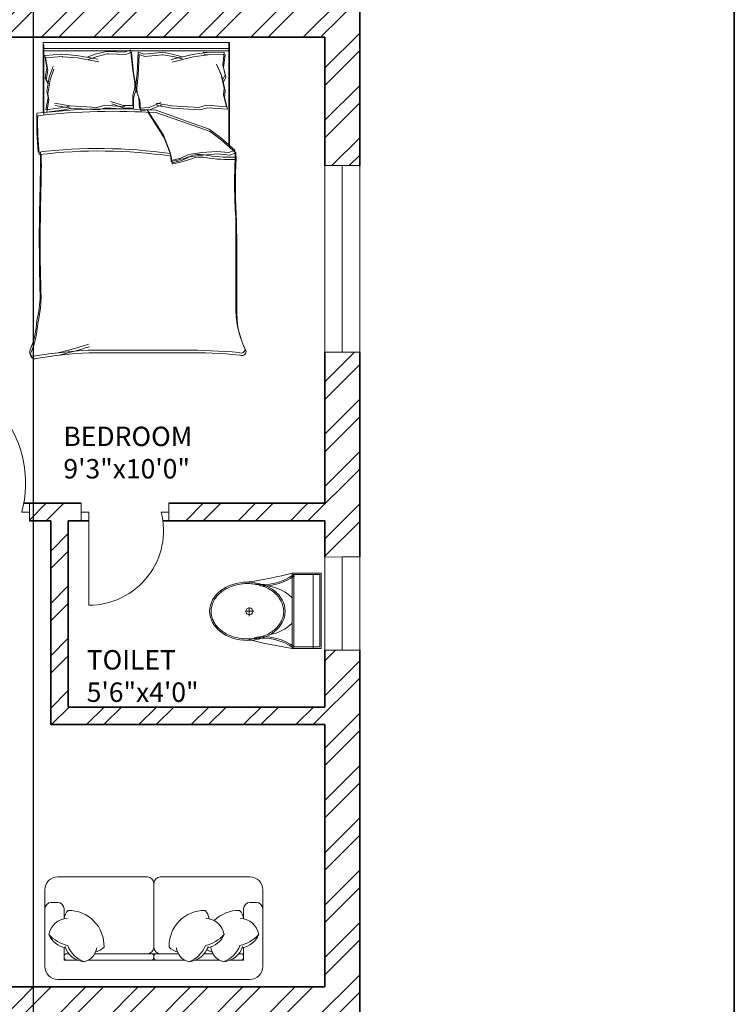
# Model space of a CAD drawing. Units: inches. Extents: x 2552 to 3217, y 1417 to 2737.
# Tile 6 of 25: x 3033 to 3217, y 1631 to 1885. Entities that reach past the tile are written whole.
import ezdxf

# ---------------------------------------------------------------- set-up
doc = ezdxf.new("R2010")
doc.units = ezdxf.units.IN
for name, color, linetype, lineweight in [('A-ANNO-DIMS', 2, 'Continuous', 18), ('A-ANNO-TTLB', 7, 'Continuous', 35), ('A-AREA-IDEN', 7, 'Continuous', 18), ('A-DOOR', 21, 'Continuous', 18), ('A-FLOR-FIXT', 8, 'Continuous', 18), ('A-FURN', 8, 'Continuous', 13), ('A-GLAZ', 161, 'Continuous', 18), ('A-WALL', 7, 'Continuous', 35), ('A-WALL-PATT', 217, 'Continuous', 13)]:
    doc.layers.add(name, color=color, linetype=linetype, lineweight=lineweight)
doc.styles.get("Standard").update_dxf_attribs({"font": 'arial.ttf'})
doc.dimstyles.get("Standard").update_dxf_attribs({"dimtxt": 0.18, "dimasz": 0.18, "dimexe": 0.18, "dimexo": 0.0625, "dimgap": 0.09, "dimtad": 0, "dimtih": 1, "dimtoh": 1, "dimdec": 4, "dimzin": 0, "dimdsep": 46, "dimtxsty": 'Standard', "dimcen": 0.09, "dimadec": 0, "dimazin": 0, "dimtfac": 1, "dimtdec": 4, "dimtofl": 0, "dimtmove": 0, "dimatfit": 3, "dimfxl": 1, "dimtolj": 1, "dimtzin": 0, "dimarcsym": 0})

# ---------------------------------------------------------------- blocks, each defined once
blk = doc.blocks.new('A$C31115884')
for p, q in [((283.1, 497.7), (223.4, 497.7)), ((257.5, 466.4), (257.5, 523.2)), ((0, 200), (0, 0)), ((520, 200), (0, 200)), ((10, 190), (10, 10)), ((510, 190), (10, 190)), ((510, 10), (510, 190)), ((520, 0), (520, 200)), ((510, 54.5), (0, 54.5)), ((10, 10), (510, 10)), ((0, 0), (520, 0))]:
    blk.add_line(p, q)
blk.add_circle((255.6, 496.4), 23.6)
for centre, radius, start, end in [((2777.7, -204.6), 2807, 165.4549, 171.71327), ((3237, 905), 2807, 188.28673, 194.5451), ((-294.5, 403.3), 364.7, 324.20913, 9.34987), ((-294.5, 403.3), 374.7, 324.20913, 9.34987), ((139.5, 406.2), 293.5, 315.84364, 2.65635), ((805.8, 403.3), 374.7, 179.20365, 215.79087), ((805.8, 403.3), 364.7, 170.65013, 215.79087), ((383.6, 406.2), 293.5, 190.27735, 224.15636)]:
    blk.add_arc(centre, radius, start, end)
blk.add_ellipse((256.2, 509.9), major_axis=(0, -260.7), ratio=0.772727)
blk.add_open_spline([(256.2, 259.2), (263.1, 259.2), (270, 259.7), (287.8, 262.3), (298.7, 265.1), (319.9, 273.1), (330.2, 278.4), (350.1, 291.1), (359.7, 298.7), (377.7, 315.9), (386.2, 325.5), (401.7, 346.6), (408.8, 358.1), (421.3, 382.5), (426.8, 395.5), (435.9, 422.4), (439.5, 436.4), (444.8, 465.1), (446.5, 479.7), (447.9, 509.2), (447.6, 524), (445, 553.3), (442.7, 567.8), (436.3, 596), (432.1, 609.7), (421.9, 636), (416, 648.6), (402.5, 672.1), (395, 683), (378.6, 703), (369.8, 712.1), (351.1, 728), (341.3, 734.8), (320.9, 746.2), (310.4, 750.7), (288.9, 757.3), (278, 759.4), (256, 761), (245, 760.6), (223.1, 757.2), (212.3, 754.3), (191.1, 746.1), (180.8, 740.7), (160.9, 727.8), (151.4, 720.1), (133.5, 702.7), (125.1, 693), (109.6, 671.7), (102.6, 660.2), (90.2, 635.7), (84.9, 622.7), (76, 595.6), (72.4, 581.6), (67.2, 552.9), (65.6, 538.2), (64.4, 508.8), (64.8, 494), (67.5, 464.7), (69.9, 450.2), (76.6, 422), (80.8, 408.3), (91.1, 382.2), (97.2, 369.7), (110.8, 346.3), (118.4, 335.4), (134.8, 315.6), (143.7, 306.7), (162.4, 290.9), (172.3, 284.2), (192.8, 273), (203.3, 268.6), (224.8, 262.2), (235.8, 260.2), (249.9, 259.3), (253, 259.2), (256.2, 259.2)], degree=3, knots=[0, 0, 0, 0, 0.110105, 0.110105, 0.285049, 0.285049, 0.459994, 0.459994, 0.634938, 0.634938, 0.809882, 0.809882, 0.984827, 0.984827, 1.159771, 1.159771, 1.334715, 1.334715, 1.50966, 1.50966, 1.684604, 1.684604, 1.859549, 1.859549, 2.034493, 2.034493, 2.209437, 2.209437, 2.384382, 2.384382, 2.559326, 2.559326, 2.73427, 2.73427, 2.909215, 2.909215, 3.084159, 3.084159, 3.259103, 3.259103, 3.434048, 3.434048, 3.608992, 3.608992, 3.783936, 3.783936, 3.958881, 3.958881, 4.133825, 4.133825, 4.30877, 4.30877, 4.483714, 4.483714, 4.658658, 4.658658, 4.833603, 4.833603, 5.008547, 5.008547, 5.183491, 5.183491, 5.358436, 5.358436, 5.53338, 5.53338, 5.708324, 5.708324, 5.883269, 5.883269, 6.058213, 6.058213, 6.233158, 6.233158, 6.283185, 6.283185, 6.283185, 6.283185])
blk = doc.blocks.new('BED-DOUBLE')
for p, q in [((3.47, 63.33), (3.47, 81.44)), ((3.47, 81.44), (51.49, 81.44)), ((3.48, 63.33), (3.48, 81.44)), ((51.27, 81.44), (51.27, 54.83)), ((51.27, 81.44), (51.27, 54.83)), ((51.49, 81.44), (51.49, 80.8)), ((3.47, 79.91), (51.27, 79.91)), ((3.48, 79.91), (51.27, 79.91)), ((3.7, 62.69), (3.7, 80.8)), ((3.7, 62.69), (3.7, 80.8)), ((3.7, 79.27), (51.49, 79.27)), ((3.7, 79.27), (51.49, 79.27)), ((16.88, 78.42), (19.77, 79.14)), ((16.88, 78.42), (19.77, 79.14)), ((19.77, 79.14), (20.09, 79.14)), ((19.77, 79.14), (20.09, 79.14)), ((20.09, 79.14), (24.54, 78.99)), ((20.09, 79.14), (24.54, 78.99)), ((24.54, 78.99), (25.98, 79.57)), ((24.54, 78.99), (25.98, 79.57)), ((24.77, 78.36), (26.21, 78.93)), ((24.77, 78.36), (26.21, 78.93)), ((25.98, 79.57), (26.56, 74.22)), ((25.98, 79.57), (26.56, 74.22)), ((26.21, 78.93), (26.79, 73.58)), ((26.21, 78.93), (26.79, 73.58)), ((27.98, 78.95), (27.73, 73.58)), ((27.98, 78.95), (27.73, 73.58)), ((29.46, 78.46), (27.98, 78.95)), ((29.46, 78.46), (27.98, 78.95)), ((33.88, 78.89), (29.46, 78.46)), ((33.88, 78.89), (29.46, 78.46)), ((34.2, 78.91), (33.88, 78.89)), ((34.2, 78.91), (33.88, 78.89)), ((37.14, 78.36), (34.2, 78.91)), ((37.14, 78.36), (34.2, 78.91)), ((45.71, 78.9), (41.91, 78.37)), ((45.71, 78.9), (41.91, 78.37)), ((50.11, 78.89), (44.71, 78.98)), ((44.71, 78.98), (45.71, 78.9)), ((50.11, 78.89), (44.71, 78.98)), ((44.71, 78.98), (45.71, 78.9)), ((50.11, 78.89), (49.73, 75.68)), ((50.11, 78.89), (49.73, 75.68)), ((51.49, 80.8), (51.49, 54.19)), ((51.49, 80.8), (51.49, 54.19)), ((3.89, 78.13), (4.47, 74.95)), ((3.89, 78.13), (4.47, 74.95)), ((3.9, 78.11), (8.18, 78.43)), ((3.9, 78.11), (8.18, 78.43)), ((4.12, 77.49), (4.7, 74.31)), ((4.12, 77.49), (4.7, 74.31)), ((4.13, 77.47), (8.41, 77.8)), ((4.13, 77.47), (8.41, 77.8)), ((8.18, 78.43), (8.28, 78.42)), ((8.18, 78.43), (8.28, 78.42)), ((8.28, 78.42), (12.11, 78.13)), ((8.28, 78.42), (12.11, 78.13)), ((8.41, 77.8), (8.51, 77.78)), ((8.41, 77.8), (8.51, 77.78)), ((8.51, 77.78), (12.34, 77.49)), ((8.51, 77.78), (12.34, 77.49)), ((12.11, 78.13), (17.6, 77.12)), ((12.11, 78.13), (17.6, 77.12)), ((12.34, 77.49), (17.83, 76.48)), ((12.34, 77.49), (17.83, 76.48)), ((14.85, 77.69), (16.88, 78.42)), ((14.85, 77.69), (16.88, 78.42)), ((15.08, 77.05), (17.11, 77.78)), ((15.08, 77.05), (17.11, 77.78)), ((17.11, 77.78), (20, 78.5)), ((17.11, 77.78), (20, 78.5)), ((20, 78.5), (20.32, 78.5)), ((20, 78.5), (20.32, 78.5)), ((20.32, 78.5), (24.77, 78.36)), ((20.32, 78.5), (24.77, 78.36)), ((28.21, 78.31), (27.96, 72.94)), ((28.21, 78.31), (27.96, 72.94)), ((29.68, 77.83), (28.21, 78.31)), ((29.68, 77.83), (28.21, 78.31)), ((34.11, 78.25), (29.68, 77.83)), ((34.11, 78.25), (29.68, 77.83)), ((34.43, 78.27), (34.11, 78.25)), ((34.43, 78.27), (34.11, 78.25)), ((37.36, 77.73), (34.43, 78.27)), ((37.36, 77.73), (34.43, 78.27)), ((41.91, 78.37), (36.49, 77.02)), ((41.91, 78.37), (36.5, 77.02)), ((42.14, 77.73), (36.72, 76.38)), ((42.14, 77.73), (36.72, 76.38)), ((39.2, 77.77), (37.14, 78.36)), ((39.2, 77.77), (37.14, 78.36)), ((39.43, 77.13), (37.36, 77.73)), ((39.43, 77.13), (37.36, 77.73)), ((45.94, 78.26), (42.14, 77.73)), ((45.94, 78.26), (42.14, 77.73)), ((50.34, 78.25), (44.94, 78.34)), ((44.94, 78.34), (45.94, 78.26)), ((50.34, 78.25), (44.94, 78.34)), ((44.94, 78.34), (45.94, 78.26)), ((50.34, 78.25), (49.96, 75.04)), ((50.34, 78.25), (49.96, 75.04)), ((4.47, 74.95), (4.04, 72.34)), ((4.47, 74.95), (4.04, 72.34)), ((4.7, 74.31), (4.27, 71.7)), ((4.7, 74.31), (4.27, 71.7)), ((5.05, 72.49), (6.06, 75.24)), ((5.05, 72.49), (6.06, 75.24)), ((5.28, 71.85), (6.29, 74.6)), ((5.28, 71.85), (6.29, 74.6)), ((26.56, 74.22), (27.14, 71.04)), ((26.56, 74.22), (27.14, 71.04)), ((26.79, 73.58), (27.37, 70.4)), ((26.79, 73.58), (27.37, 70.4)), ((27.73, 73.58), (27.35, 70.37)), ((27.73, 73.58), (27.35, 70.37)), ((49.31, 73.19), (48.13, 75.86)), ((49.31, 73.19), (48.13, 75.86)), ((49.54, 72.55), (48.36, 75.23)), ((49.54, 72.55), (48.36, 75.23)), ((49.73, 75.68), (50.33, 73.1)), ((49.73, 75.68), (50.33, 73.1)), ((49.96, 75.04), (50.56, 72.47)), ((49.96, 75.04), (50.56, 72.47)), ((4.04, 72.34), (4.62, 71.33)), ((4.04, 72.34), (4.62, 71.33)), ((4.27, 71.7), (4.85, 70.69)), ((4.27, 71.7), (4.85, 70.69)), ((4.47, 68.87), (5.05, 72.49)), ((4.47, 68.87), (5.05, 72.49)), ((4.7, 68.23), (5.28, 71.85)), ((4.7, 68.23), (5.28, 71.85)), ((27.14, 71.04), (27.14, 69.74)), ((27.14, 71.04), (27.14, 69.74)), ((27.96, 72.94), (27.58, 69.73)), ((27.96, 72.94), (27.58, 69.73)), ((50.11, 69.61), (49.31, 73.19)), ((50.11, 69.61), (49.31, 73.19)), ((50.34, 68.98), (49.54, 72.55)), ((50.34, 68.98), (49.54, 72.55)), ((50.33, 73.1), (49.81, 72.06)), ((50.33, 73.1), (49.81, 72.06)), ((50.56, 72.47), (50.04, 71.42)), ((50.56, 72.47), (50.04, 71.42)), ((4.76, 67.28), (4.47, 68.87)), ((4.76, 67.28), (4.47, 68.87)), ((27.14, 69.74), (26.56, 67.86)), ((27.14, 69.74), (26.56, 67.86)), ((27.37, 69.1), (26.79, 67.22)), ((27.37, 69.1), (26.79, 67.22)), ((27.35, 70.37), (27.44, 69.07)), ((27.35, 70.37), (27.44, 69.07)), ((27.37, 70.4), (27.37, 69.1)), ((27.37, 70.4), (27.37, 69.1)), ((27.44, 69.07), (28.13, 67.23)), ((27.44, 69.07), (28.13, 67.23)), ((27.58, 69.73), (27.66, 68.43)), ((27.58, 69.73), (27.66, 68.43)), ((49.92, 68.01), (50.11, 69.61)), ((49.92, 68.01), (50.11, 69.61)), ((50.15, 67.37), (50.34, 68.98)), ((50.15, 67.37), (50.34, 68.98)), ((4.18, 64.1), (4.76, 67.28)), ((4.18, 64.1), (4.76, 67.28)), ((4.41, 63.46), (4.99, 66.64)), ((4.41, 63.46), (4.99, 66.64)), ((4.99, 66.64), (4.7, 68.23)), ((4.99, 66.64), (4.7, 68.23)), ((24.1, 65.18), (20.96, 66.27)), ((24.1, 65.18), (20.96, 66.27)), ((26.56, 67.86), (26.56, 65.18)), ((26.56, 67.86), (26.56, 65.18)), ((26.79, 67.22), (26.79, 64.54)), ((26.79, 67.22), (26.79, 64.54)), ((27.66, 68.43), (28.36, 66.59)), ((27.66, 68.43), (28.36, 66.59)), ((28.13, 67.23), (28.3, 64.55)), ((28.13, 67.23), (28.3, 64.55)), ((28.36, 66.59), (28.53, 63.91)), ((28.36, 66.59), (28.53, 63.91)), ((30.75, 64.7), (33.82, 65.99)), ((30.75, 64.7), (33.82, 65.99)), ((50.7, 64.87), (49.92, 68.01)), ((50.7, 64.87), (49.92, 68.01)), ((50.93, 64.23), (50.15, 67.37)), ((50.93, 64.23), (50.15, 67.37)), ((9.28, 64.83), (4.18, 64.1)), ((9.28, 64.83), (4.18, 64.1)), ((9.51, 64.19), (4.41, 63.46)), ((9.51, 64.19), (4.41, 63.46)), ((6.38, 65.81), (10.41, 65.15)), ((6.38, 65.81), (10.41, 65.15)), ((6.61, 65.18), (10.64, 64.51)), ((6.61, 65.18), (10.64, 64.51)), ((10.41, 65.15), (9.28, 64.83)), ((10.41, 65.15), (9.28, 64.83)), ((10.64, 64.51), (9.51, 64.19)), ((10.64, 64.51), (9.51, 64.19)), ((10.41, 65.15), (17.42, 64.72)), ((10.41, 65.15), (17.42, 64.72)), ((10.64, 64.51), (17.65, 64.08)), ((10.64, 64.51), (17.65, 64.08)), ((17.42, 64.72), (19.38, 65.27)), ((17.42, 64.72), (19.38, 65.27)), ((17.65, 64.08), (19.61, 64.63)), ((17.65, 64.08), (19.61, 64.63)), ((19.38, 65.27), (24.52, 64.87)), ((19.38, 65.27), (24.52, 64.87)), ((19.61, 64.63), (24.74, 64.23)), ((19.61, 64.63), (24.74, 64.23)), ((24.33, 64.54), (21.19, 65.63)), ((24.33, 64.54), (21.19, 65.63)), ((26.56, 65.18), (24.1, 65.18)), ((26.56, 65.18), (24.1, 65.18)), ((26.79, 64.54), (24.33, 64.54)), ((26.79, 64.54), (24.33, 64.54)), ((28.3, 64.55), (30.75, 64.7)), ((28.3, 64.55), (30.75, 64.7)), ((28.53, 63.91), (30.98, 64.06)), ((28.53, 63.91), (30.98, 64.06)), ((30.26, 64.06), (34.45, 57.57)), ((30.26, 64.06), (34.45, 57.57)), ((30.49, 63.42), (34.68, 56.93)), ((30.49, 63.42), (34.68, 56.93)), ((30.98, 64.06), (34.05, 65.35)), ((30.98, 64.06), (34.05, 65.35)), ((40.64, 61.13), (32.31, 64.06)), ((40.64, 61.13), (32.31, 64.06)), ((40.87, 60.49), (32.53, 63.42)), ((40.87, 60.49), (32.53, 63.42)), ((32.56, 65.81), (36.6, 65.15)), ((32.56, 65.81), (36.6, 65.15)), ((32.79, 65.18), (36.82, 64.51)), ((32.79, 65.18), (36.82, 64.51)), ((36.6, 65.15), (43.61, 64.72)), ((36.6, 65.15), (43.61, 64.72)), ((36.82, 64.51), (43.83, 64.08)), ((36.82, 64.51), (43.83, 64.08)), ((43.61, 64.72), (45.57, 65.27)), ((43.61, 64.72), (45.57, 65.27)), ((43.83, 64.08), (45.79, 64.63)), ((43.83, 64.08), (45.79, 64.63)), ((45.57, 65.27), (50.7, 64.87)), ((45.57, 65.27), (50.7, 64.87)), ((45.79, 64.63), (50.93, 64.23)), ((45.79, 64.63), (50.93, 64.23)), ((46.22, 59.11), (40.64, 61.13)), ((46.22, 59.11), (40.64, 61.13)), ((46.45, 58.48), (40.87, 60.49)), ((46.45, 58.48), (40.87, 60.49)), ((49.16, 56.95), (46.22, 59.11)), ((49.16, 56.95), (46.22, 59.11)), ((49.39, 56.31), (46.45, 58.48)), ((49.39, 56.31), (46.45, 58.48)), ((34.45, 57.57), (36.15, 53.08)), ((34.45, 57.57), (36.15, 53.08)), ((34.68, 56.93), (36.38, 52.44)), ((34.68, 56.93), (36.38, 52.44)), ((52.87, 53.7), (49.16, 56.95)), ((52.87, 53.7), (49.16, 56.95)), ((53.1, 53.06), (49.39, 56.31)), ((53.1, 53.06), (49.39, 56.31)), ((44.36, 53.08), (48.23, 53.39)), ((44.36, 53.08), (48.23, 53.39)), ((48.23, 53.39), (51.33, 53.08)), ((48.23, 53.39), (51.33, 53.08)), ((51.33, 53.08), (52.87, 53.7)), ((51.33, 53.08), (52.87, 53.7)), ((52.95, 51.95), (52.87, 53.7, 3.87)), ((52.95, 51.95), (52.87, 53.7, 3.87)), ((36.15, 53.08), (36.46, 51.07)), ((36.15, 53.08), (36.46, 51.07)), ((36.38, 52.44), (36.69, 50.43)), ((36.38, 52.44), (36.69, 50.43)), ((36.46, 51.07), (38.94, 51.69)), ((36.46, 51.07), (38.94, 51.69)), ((36.69, 50.43), (39.17, 51.05)), ((36.69, 50.43), (39.17, 51.05)), ((38.94, 51.69), (40.95, 52.61)), ((38.94, 51.69), (40.95, 52.61)), ((39.17, 51.05), (41.18, 51.97)), ((39.17, 51.05), (41.18, 51.97)), ((40.95, 52.61), (44.36, 53.08)), ((40.95, 52.61), (44.36, 53.08)), ((41.18, 51.97), (44.59, 52.44)), ((41.18, 51.97), (44.59, 52.44)), ((44.59, 52.44), (48.46, 52.75)), ((44.59, 52.44), (48.46, 52.75)), ((48.46, 52.75), (51.56, 52.44)), ((48.46, 52.75), (51.56, 52.44)), ((51.56, 52.44), (53.1, 53.06)), ((51.56, 52.44), (53.1, 53.06)), ((53.18, 51.31), (53.1, 53.06, 3.87)), ((53.18, 51.31), (53.1, 53.06, 3.87)), ((15.06, 2.2), (39.68, 2.2)), ((15.06, 2.2), (39.68, 2.2)), ((15.29, 1.56), (39.91, 1.56)), ((15.29, 1.56), (39.91, 1.56))]:
    blk.add_line(p, q)
for centre, radius, start, end in [((21.36, -100.61), 164.97, 86.0865, 96.7821), ((21.36, -100.61), 164.97, 86.0865, 96.7821), ((21.59, -101.25), 164.97, 86.0865, 96.7821), ((21.59, -101.25), 164.97, 86.0865, 96.7821), ((85.16, 61.35), 83.31, 178.7218, 185.604), ((85.16, 61.35), 83.31, 178.7218, 185.604), ((85.39, 60.71), 83.31, 178.7218, 185.604), ((85.39, 60.71), 83.31, 178.7218, 185.604), ((17.76, -74.87), 129.02, 81.7845, 96.9006), ((17.76, -74.87), 129.02, 81.7845, 96.9006), ((17.98, -75.51), 129.02, 81.7845, 96.9006), ((17.98, -75.51), 129.02, 81.7845, 96.9006), ((-167.31, 50.27), 170.11, 358.4762, 1.0082), ((-167.31, 50.27), 170.11, 358.4762, 1.0082), ((-167.08, 49.63), 170.11, 358.4762, 1.0082), ((-167.08, 49.63), 170.11, 358.4762, 1.0082), ((36.64, 51), 0.185, 160.2464, 271.1377), ((36.64, 51), 0.185, 160.2464, 271.1377), ((31.15, 79.96), 29.65, 280.6617, 289.8806), ((31.15, 79.96), 29.65, 280.6617, 289.8806), ((31.38, 79.32), 29.65, 280.6617, 289.8806), ((31.38, 79.32), 29.65, 280.6617, 289.8806), ((43.74, 46.38), 6.22, 78.6608, 113.7384), ((43.74, 46.38), 6.22, 78.6608, 113.7384), ((43.97, 45.74), 6.22, 78.6608, 113.7384), ((43.97, 45.74), 6.22, 78.6608, 113.7384), ((51.33, 88.1), 36.18, 259.8763, 272.5657), ((51.33, 88.1), 36.18, 259.8763, 272.5657), ((51.56, 87.46), 36.18, 259.8763, 272.5657), ((51.56, 87.46), 36.18, 259.8763, 272.5657), ((182.27, 45.13), 129.5, 176.9791, 183.8365), ((182.27, 45.13), 129.5, 176.9791, 183.8365), ((182.49, 44.49), 129.5, 176.9791, 183.8365), ((182.49, 44.49), 129.5, 176.9791, 183.8365), ((36.86, 50.36), 0.185, 160.2464, 271.1377), ((36.86, 50.36), 0.185, 160.2464, 271.1377), ((484.82, 30.83), 482.31, 178.2277, 181.7185), ((484.82, 30.83), 482.31, 178.2277, 181.7185), ((485.05, 30.19), 482.31, 178.2277, 181.7185), ((485.05, 30.19), 482.31, 178.2277, 181.7185), ((-4508.74, 13.62), 4561.86, 0.00217, 0.28689), ((-4508.74, 13.62), 4561.86, 0.00217, 0.28689), ((-4508.51, 12.98), 4561.86, 0.00217, 0.28689), ((-4508.52, 12.98), 4561.86, 0.00217, 0.28689), ((-26.9, 16.93), 29.63, 346.0648, 358.9113), ((-26.9, 16.93), 29.63, 346.0648, 358.9113), ((-26.67, 16.29), 29.63, 346.0648, 358.9113), ((-26.67, 16.29), 29.63, 346.0648, 358.9113), ((76.16, 12.78), 23.07, 177.4714, 206.4681), ((76.16, 12.78), 23.07, 177.4714, 206.4681), ((76.39, 12.14), 23.07, 177.4714, 206.4681), ((76.39, 12.14), 23.07, 177.4714, 206.4681), ((-21.66, 11.17), 23.56, 337.9751, 356.652), ((-21.66, 11.17), 23.56, 337.9751, 356.652), ((-21.43, 10.53), 23.56, 337.9751, 356.652), ((-21.43, 10.53), 23.56, 337.9751, 356.652), ((-17.22, 105.16), 106.46, 283.3832, 287.7053), ((-17.22, 105.16), 106.46, 283.3832, 287.7053), ((-16.99, 104.52), 106.46, 283.3832, 287.7053), ((-16.99, 104.52), 106.46, 283.3832, 287.7053), ((1.09, 1.73), 1.09, 146.1736, 293.4781), ((1.09, 1.73), 1.09, 146.1736, 293.4781), ((1.32, 1.09), 1.09, 146.1736, 293.4781), ((1.32, 1.09), 1.09, 146.1736, 293.4781), ((21.43, -119.39), 121.76, 92.9958, 99.4091), ((21.43, -119.39), 121.76, 92.9958, 99.4091), ((21.66, -120.03), 121.76, 92.9958, 99.4091), ((21.65, -120.03), 121.76, 92.9958, 99.4091), ((41.15, -130.83), 133.04, 84.4998, 90.6351), ((41.15, -130.83), 133.04, 84.4998, 90.6351), ((41.38, -131.47), 133.04, 84.4998, 90.6351), ((41.38, -131.47), 133.04, 84.4998, 90.6351), ((54.41, 2.57), 1.1, 242.6588, 356.02), ((54.41, 2.57), 1.1, 242.6588, 356.02), ((54.64, 1.93), 1.1, 242.6588, 356.02), ((54.64, 1.93), 1.1, 242.6588, 356.02)]:
    blk.add_arc(centre, radius, start, end)
blk = doc.blocks.new('WIN-48')
for p, q in [((4.5, 48), (0, 48)), ((0, 48), (9, 48)), ((0, 48), (0, 0)), ((4.5, 0), (4.5, 48)), ((9, 48), (9, 0)), ((0, 0), (9, 0)), ((9, 0), (4.5, 0))]:
    blk.add_line(p, q)
blk = doc.blocks.new('*D57')
at = {"layer": 'A-ANNO-DIMS', "color": 0, "lineweight": -2, "transparency": 16777216}
for p, q in [((3004.08, 2515.95), (3004.08, 1482.53)), ((3036.34, 2515.95), (3036.34, 1482.53)), ((3004.26, 1482.71), (3019.75, 1482.71)), ((3036.16, 1482.71), (3020.68, 1482.71))]:
    blk.add_line(p, q, dxfattribs=at)
at = {"layer": 'A-ANNO-DIMS', "color": 0, "transparency": 16777216}
for points in [[(3004.26, 1482.74), (3004.26, 1482.68), (3004.08, 1482.71)], [(3036.16, 1482.74), (3036.16, 1482.68), (3036.34, 1482.71)]]:
    blk.add_solid(points, dxfattribs=at)
at = {"layer": 'Defpoints', "color": 0, "transparency": 16777216}
for p in [(3004.08, 2516.01), (3036.34, 2516.01), (3036.34, 1482.71)]:
    blk.add_point(p, dxfattribs=at)
at = {"layer": 'A-ANNO-DIMS', "color": 0, "transparency": 16777216, "insert": (3020.21, 1482.71), "char_height": 0.18, "attachment_point": 5}
blk.add_mtext('\\A1;32.255', dxfattribs=at)

msp = doc.modelspace()

# ---------------------------------------------------------------- hatches: boundary and pattern name
at = {"layer": 'A-WALL-PATT'}
h = msp.add_hatch(dxfattribs=at)
h.set_pattern_fill('ANSI32', color=256)
h.paths.add_polyline_path([(2756.676, 2649.5125), (2637.3535, 2649.5125), (2637.3535, 2617.9626), (2641.8535, 2617.9626), (2646.3535, 2617.9626), (2646.3535, 2640.5125), (2724.3535, 2640.5125), (2724.3535, 2520.5125), (2720.299, 2520.5125), (2720.299, 2516.0125), (2733.4075, 2516.0125), (2733.4075, 2518.2213), (2733.4075, 2520.5125), (2728.8535, 2520.5125), (2728.8535, 2640.5125), (2756.676, 2640.5125)])
h.paths.add_polyline_path([(2848.8535, 2649.5125), (2804.676, 2649.5125), (2804.676, 2640.5125), (2839.8535, 2640.5125), (2839.8535, 2598.3517), (2848.8535, 2598.3517)])
h.paths.add_polyline_path([(2646.3535, 2516.0125), (2697.9593, 2516.0125), (2697.9593, 2518.2625), (2697.9593, 2520.5125), (2646.3535, 2520.5125), (2646.3535, 2581.9626), (2637.3535, 2581.9626), (2637.3535, 2364.3298), (2646.3535, 2364.3298), (2646.3535, 2387.0125), (2724.3535, 2387.0125), (2724.3535, 2267.0125), (2721.0443, 2267.0125), (2721.0443, 2262.5125), (2733.7854, 2262.5125), (2733.7854, 2264.7625), (2733.7854, 2267.0125), (2728.8535, 2267.0125), (2728.8535, 2387.0125), (2839.8535, 2387.0125), (2839.8535, 2363.8387), (2848.8535, 2363.8387), (2848.8535, 2403.7415), (2844.3535, 2403.7415), (2839.8535, 2403.7415), (2839.8535, 2396.0125), (2646.3535, 2396.0125)])
h.paths.add_polyline_path([(2848.8535, 2550.3517), (2844.3535, 2550.3517), (2839.8535, 2550.3517), (2839.8535, 2520.5125), (2801.9195, 2520.5125), (2801.9195, 2518.2625), (2801.9195, 2516.0125), (2839.8535, 2516.0125), (2839.8535, 2507.5813), (2848.8535, 2507.5813)], flags=17)
h.paths.add_polyline_path([(2848.8535, 2483.5813), (2844.3535, 2483.5813), (2839.8535, 2483.5813), (2839.8535, 2468.0125), (2773.8535, 2468.0125), (2773.8535, 2516.0125), (2778.1336, 2516.0125), (2778.1336, 2520.5125), (2766.696, 2520.5125), (2766.696, 2518.2625), (2766.696, 2516.0125), (2769.3535, 2516.0125), (2769.3535, 2463.5125), (2839.8535, 2463.5125), (2839.8535, 2431.0782), (2848.8535, 2431.0782)], flags=17)
h.paths.add_polyline_path([(2917.8535, 2569.2764), (2913.3535, 2569.2764), (2908.8535, 2569.2764), (2908.8535, 2433.001), (2917.8535, 2433.001), (2917.8535, 2516.0125), (2967.486, 2516.0125), (2967.486, 2520.5125), (2917.8535, 2520.5125)])
h.paths.add_polyline_path([(3000.3535, 2640.5125), (2995.8535, 2640.5125), (2995.8535, 2520.5125), (2990.688, 2520.5125), (2990.688, 2516.0125), (3004.0844, 2516.0125), (3004.0844, 2518.2625), (3004.0844, 2520.5125), (3000.3535, 2520.5125)])
h.paths.add_polyline_path([(3120.3535, 2561.3689), (3115.8535, 2561.3689), (3111.3535, 2561.3689), (3111.3535, 2520.5125), (3070.9814, 2520.5125), (3070.9814, 2518.2625), (3070.9814, 2516.0125), (3111.3535, 2516.0125), (3111.3535, 2505.1841), (3120.3535, 2505.1841)])
h.paths.add_polyline_path([(3120.3535, 2481.1841), (3115.8535, 2481.1841), (3111.3535, 2481.1841), (3111.3535, 2468.0125), (3045.3535, 2468.0125), (3045.3535, 2516.0125), (3048.9787, 2516.0125), (3048.9787, 2520.5125), (3036.3395, 2520.5125), (3036.3395, 2516.0125), (3040.8535, 2516.0125), (3040.8535, 2463.5125), (3111.3535, 2463.5125), (3111.3535, 2396.0125), (2917.8535, 2396.0125), (2917.8535, 2403.4124), (2913.3535, 2403.4124), (2908.8535, 2403.4124), (2908.8535, 2182.5756), (2917.8535, 2182.5756), (2917.8535, 2262.5125), (2968.001, 2262.5125), (2968.001, 2264.7625), (2968.001, 2267.0125), (2917.8535, 2267.0125), (2917.8535, 2387.0125), (3111.3535, 2387.0125), (3111.3535, 2352.2435), (3120.3535, 2352.2435)])
h.paths.add_polyline_path([(3120.3535, 2304.2435), (3115.8535, 2304.2435), (3111.3535, 2304.2435), (3111.3535, 2267.0125), (3073.8616, 2267.0125), (3073.8616, 2264.7625), (3073.8616, 2262.5125), (3111.3535, 2262.5125), (3111.3535, 2252.376), (3120.3535, 2252.376)], flags=17)
h.paths.add_polyline_path([(3120.3535, 2228.376), (3115.8535, 2228.376), (3111.3535, 2228.376), (3111.3535, 2214.5125), (3045.3535, 2214.5125), (3045.3535, 2262.5125), (3049.3096, 2262.5125), (3049.3096, 2267.0125), (3035.0125, 2267.0125), (3035.0125, 2262.5125), (3040.8535, 2262.5125), (3040.8535, 2210.0125), (3111.3535, 2210.0125), (3111.3535, 2142.5125), (2917.8535, 2142.5125), (2917.8535, 2150.2408), (2913.3535, 2150.2408), (2908.8535, 2150.2408), (2908.8535, 1924.9905), (2917.8535, 1924.9905), (2917.8535, 2009.0125), (2971.959, 2009.0125), (2971.959, 2011.2625), (2971.959, 2013.5125), (2917.8535, 2013.5125), (2917.8535, 2133.5125), (2995.8535, 2133.5125), (2995.8535, 2013.5125), (2992.1797, 2013.5125), (2992.1797, 2009.0125), (3004.3344, 2009.0125), (3004.3344, 2011.2625), (3004.3344, 2013.5125), (3000.3535, 2013.5125), (3000.3535, 2133.5125), (3111.3535, 2133.5125), (3111.3535, 2115.0291), (3120.3535, 2115.0291)])
h.paths.add_polyline_path([(3000.3535, 2387.0125), (2995.8535, 2387.0125), (2995.8535, 2267.0125), (2991.3326, 2267.0125), (2991.3326, 2262.5125), (3004.1044, 2262.5125), (3004.1044, 2264.7625), (3004.1044, 2267.0125), (3000.3535, 2267.0125)], flags=17)
h.paths.add_polyline_path([(3120.3535, 1973.2388), (3115.8535, 1973.2388), (3111.3535, 1973.2388), (3111.3535, 1961.0125), (3045.3535, 1961.0125), (3045.3535, 2009.0125), (3048.9101, 2009.0125), (3048.9101, 2013.5125), (3037.105, 2013.5125), (3037.105, 2011.2625), (3037.105, 2009.0125), (3040.8535, 2009.0125), (3040.8535, 1956.5125), (3111.3535, 1956.5125), (3111.3535, 1889.0125), (2917.8535, 1889.0125), (2917.8535, 1895.7215), (2913.3535, 1895.7215), (2908.8535, 1895.7215), (2908.8535, 1844.2217), (2917.8535, 1844.2217), (2917.8535, 1880.0125), (3111.3535, 1880.0125), (3111.3535, 1846.9541), (3120.3535, 1846.9541)])
h.paths.add_polyline_path([(3120.3535, 2067.0291), (3111.3535, 2067.0291), (3111.3535, 2013.5125), (3071.3001, 2013.5125), (3071.3001, 2009.0125), (3111.3535, 2009.0125), (3111.3535, 1997.2388), (3120.3535, 1997.2388)], flags=0)
h.paths.add_polyline_path([(3120.3535, 1798.9541), (3115.8535, 1798.9541), (3111.3535, 1798.9541), (3111.3535, 1760.0125), (3071.2497, 1760.0125), (3071.2497, 1757.7625), (3071.2497, 1755.5125), (3111.3535, 1755.5125), (3111.3535, 1746.162), (3120.3535, 1746.2478)])
h.paths.add_polyline_path([(3120.3535, 1722.2049), (3111.3535, 1722.2049), (3111.3535, 1707.5125), (3045.3535, 1707.5125), (3045.3535, 1755.5125), (3048.6624, 1755.5125), (3048.6624, 1760.0125), (3035.3703, 1760.0125), (3035.3703, 1755.5125), (3040.8535, 1755.5125), (3040.8535, 1703.0125), (3111.3535, 1703.0125), (3111.3535, 1635.5125), (2917.8535, 1635.5125), (2917.8535, 1643.1366), (2913.3535, 1643.1366), (2908.8535, 1643.1366), (2908.8535, 1626.5125), (3120.3535, 1626.5125)])
h.paths.add_polyline_path([(2917.8535, 1755.5125), (2973.2287, 1755.5125), (2973.2287, 1757.7625), (2973.2287, 1760.0125), (2917.8535, 1760.0125), (2917.8535, 1808.2217), (2913.3535, 1808.2217), (2908.8535, 1808.2217), (2908.8535, 1676.1665), (2917.8535, 1676.1665)])
h.paths.add_polyline_path([(3000.3535, 1880.0125), (2995.8535, 1880.0125), (2995.8535, 1760.0125), (2992.9329, 1760.0125), (2992.9329, 1755.5125), (3003.8766, 1755.5125), (3003.8766, 1757.7625), (3003.8766, 1760.0125), (3000.3535, 1760.0125)])
h.paths.add_polyline_path([(2848.8535, 1896.6971), (2844.3535, 1896.6971), (2839.8535, 1896.6971), (2839.8535, 1889.0125), (2646.3535, 1889.0125), (2646.3535, 2009.0125), (2700.5253, 2009.0125), (2700.5253, 2011.2625), (2700.5253, 2013.5125), (2646.3535, 2013.5125), (2646.3535, 2053.1812), (2641.8535, 2053.1812), (2637.3535, 2053.1812), (2637.3535, 1836.254), (2646.3535, 1836.254), (2646.3535, 1880.0125), (2724.3535, 1880.0125), (2724.3535, 1760.0125), (2721.2473, 1760.0125), (2721.2473, 1755.5125), (2731.9187, 1755.5125), (2731.9187, 1757.7625), (2731.9187, 1760.0125), (2728.8535, 1760.0125), (2728.8535, 1880.0125), (2839.8535, 1880.0125), (2839.8535, 1840.3813), (2848.8535, 1840.3813)])
h.paths.add_polyline_path([(2848.8535, 1792.3813), (2844.3535, 1792.3813), (2839.8535, 1792.3813), (2839.8535, 1760.0125), (2797.8845, 1760.0125), (2797.8845, 1755.5125), (2839.8535, 1755.5125), (2839.8535, 1743.3688), (2844.3535, 1743.3688), (2848.8535, 1743.3688)], flags=0)
h.paths.add_polyline_path([(2848.8535, 1719.3688), (2844.3535, 1719.3688), (2839.8535, 1719.3688), (2839.8535, 1707.5125), (2773.8535, 1707.5125), (2773.8535, 1755.5125), (2777.716, 1755.5125), (2777.716, 1760.0125), (2760.9247, 1760.0125), (2760.9247, 1757.9721), (2760.9247, 1755.5125), (2769.3535, 1755.5125), (2769.3535, 1703.0125), (2839.8535, 1703.0125), (2839.8535, 1673.0277), (2848.8535, 1672.9407)], flags=0)
h.paths.add_polyline_path([(2646.3535, 1755.5125), (2702.9171, 1755.5125), (2702.9171, 1757.7625), (2702.9171, 1760.0125), (2646.3535, 1760.0125), (2646.3535, 1800.254), (2641.8535, 1800.254), (2637.3535, 1800.254), (2637.3535, 1626.5125), (2848.8535, 1626.5125), (2848.8535, 1643.1187), (2844.3535, 1643.1187), (2839.8535, 1643.1187), (2839.8535, 1635.5125), (2646.3535, 1635.5125)])
h.paths.add_polyline_path([(2848.8535, 2148.8427), (2844.3535, 2148.8427), (2839.8535, 2148.8427), (2839.8535, 2142.5125), (2646.3535, 2142.5125), (2646.3535, 2262.5125), (2701.3562, 2262.5125), (2701.3562, 2264.7625), (2701.3562, 2267.0125), (2646.3535, 2267.0125), (2646.3535, 2328.3298), (2637.3535, 2328.3298), (2637.3535, 2089.1812), (2646.3535, 2089.1812), (2646.3535, 2133.5125), (2839.8535, 2133.5125), (2839.8535, 2097.5966), (2848.8535, 2097.5966)])
h.paths.add_polyline_path([(2728.8535, 2133.5125), (2724.3535, 2133.5125), (2724.3535, 2013.5125), (2719.6039, 2013.5125), (2719.6039, 2009.0125), (2732.5784, 2009.0125), (2732.5784, 2011.2625), (2732.5784, 2013.5125), (2728.8535, 2013.5125)])
h.paths.add_polyline_path([(2848.8535, 1970.0557), (2844.3535, 1970.0557), (2839.8535, 1970.0557), (2839.8535, 1961.0125), (2773.8535, 1961.0125), (2773.8535, 2009.0125), (2777.3388, 2009.0125), (2777.3388, 2013.5125), (2764.7681, 2013.5125), (2764.7681, 2009.0125), (2769.3535, 2009.0125), (2769.3535, 1956.5125), (2839.8535, 1956.5125), (2839.8535, 1924.7199), (2848.8535, 1924.7199)], flags=17)
h.paths.add_polyline_path([(2848.8535, 2049.5966), (2844.3535, 2049.5966), (2839.8535, 2049.5966), (2839.8535, 2013.5125), (2798.198, 2013.5125), (2798.198, 2011.2625), (2798.198, 2009.0125), (2839.8535, 2009.0125), (2839.8535, 1994.0557), (2848.8535, 1994.0557)], flags=17)
h.paths.add_polyline_path([(2848.8535, 2315.8387), (2839.8535, 2315.8387), (2839.8535, 2267.0125), (2799.3375, 2267.0125), (2799.3375, 2264.7625), (2799.3375, 2262.5125), (2839.8535, 2262.5125), (2839.8535, 2253.2843), (2848.8535, 2253.2843)], flags=17)
h.paths.add_polyline_path([(2848.8535, 2229.2843), (2839.8535, 2229.2843), (2839.8535, 2177.6936), (2848.8535, 2177.6936)], flags=17)
h.paths.add_polyline_path([(2839.8535, 2214.5125), (2773.8535, 2214.5125), (2773.8535, 2262.5125), (2777.6984, 2262.5125), (2777.6984, 2267.0125), (2763.8226, 2267.0125), (2763.8226, 2262.5125), (2769.3535, 2262.5125), (2769.3535, 2210.0125), (2839.8535, 2210.0125)], flags=17)
h.paths.add_polyline_path([(3050.32, 2520.2817), (3088.9114, 2520.2817), (3088.9114, 2538.939), (3050.32, 2538.939)], flags=9)

# ---------------------------------------------------------------- linework, layer by layer
at = {"layer": 'A-ANNO-TTLB'}
msp.add_lwpolyline([(2552.473, 2736.5692), (3216.7862, 2736.5692), (3216.7862, 1416.6914), (2552.473, 1416.6914)], close=True, dxfattribs=at)
at = {"layer": 'A-DOOR'}
for p, q in [((3035.3703, 1760.0125), (3035.3703, 1755.5125)), ((3048.6624, 1755.5125), (3048.6624, 1760.0125)), ((3048.6624, 1760.0125), (3048.6624, 1757.7625)), ((3071.2497, 1755.5125), (3071.2497, 1760.0125)), ((3071.2497, 1760.0125), (3071.2497, 1757.7625)), ((3035.3703, 1757.7625), (3033.3703, 1757.7625)), ((3035.3703, 1755.5125), (3035.3703, 1757.7625)), ((3048.6624, 1757.7625), (3050.6624, 1757.7625)), ((3050.6624, 1757.7625), (3050.6624, 1733.7625)), ((3071.2497, 1757.7625), (3069.2497, 1757.7625))]:
    msp.add_line(p, q, dxfattribs=at)
for centre, radius, start, end in [((3005.8766, 1765.2638), 28.4987, 344.739016, 90), ((3050.6624, 1752.9602), 19.1977, 270, 14.486391)]:
    msp.add_arc(centre, radius, start, end, dxfattribs=at)
at = {"layer": 'A-FURN', "ltscale": 0.03}
msp.add_lwpolyline([(3065.7199, 1663.8268, -0.41421356), (3067.3695, 1662.1772, -0.41421356), (3069.0191, 1663.8268), (3092.113, 1663.8268, -0.41421356), (3095.4121, 1660.5277), (3095.4121, 1640.7329, -0.41421356), (3092.113, 1637.4338), (3042.6261, 1637.4338, -0.41421356), (3039.3269, 1640.7329), (3039.3269, 1660.5277, -0.41421356), (3042.6261, 1663.8268), (3065.7199, 1663.8268, -0.41421356), (3067.3695, 1662.1772, -0.41421356), (3069.0191, 1663.8268)], format="xyb", dxfattribs=at)
at = {"layer": 'A-FURN'}
for points in [[(3065.7199, 1644.032, 0.41421356), (3067.3695, 1645.6816), (3067.3695, 1662.1772, 0.41421356)], [(3069.0191, 1644.032, -0.41421356), (3067.3695, 1645.6816), (3067.3695, 1662.1772, -0.41421356)], [(3039.3269, 1655.579, -0.41421356), (3040.9765, 1657.2285), (3042.6261, 1657.2285, -0.41421356), (3044.2756, 1655.579), (3044.2756, 1653.0232)], [(3090.4634, 1653.0232), (3090.4634, 1655.579, -0.41421356), (3092.113, 1657.2285), (3093.7625, 1657.2285, -0.41421356), (3095.4121, 1655.579)], [(3045.1034, 1653.123, 0.35677236), (3040.3768, 1648.9651, 0.24954205), (3044.6596, 1645.5386, -9.61688035)], [(3044.272, 1653.0225, -0.16554063), (3045.2925, 1655.202, -0.42598917), (3054.5568, 1645.7522, -0.12152332), (3052.3576, 1644.4497, 7.11546429)], [(3081.5808, 1653.0225, 0.16554063), (3080.5604, 1655.202, 0.42598917), (3071.2961, 1645.7522, 0.12152332), (3073.4953, 1644.4497, -7.11546429)], [(3080.7494, 1653.123, -0.35677236), (3085.4761, 1648.9651, -0.24954205), (3081.1933, 1645.5386, 9.61688035)], [(3090.467, 1653.0225, 0.16554063), (3089.4465, 1655.202, 0.20023115), (3082.8983, 1652.5475, 0.12152332)], [(3089.6356, 1653.123, -0.35677236), (3094.3622, 1648.9651, -0.24954205), (3090.0794, 1645.5386, 9.61688035)], [(3040.3768, 1648.9651, 0.14772988), (3045.198, 1646.1302, 0.21334276), (3049.452, 1641.9723, 0.17866181)], [(3085.4761, 1648.9651, -0.14772988), (3080.6549, 1646.1302, -0.21334276), (3076.4009, 1641.9723, -0.17866181)], [(3094.3622, 1648.9651, -0.14772988), (3089.541, 1646.1302, -0.21334276), (3085.287, 1641.9723, -0.17866181)], [(3044.5319, 1645.9042, 0.30666349), (3049.452, 1641.9723, 0.30632997), (3052.6661, 1645.5632, -0.87284716)], [(3065.7199, 1644.032, 0.41421356), (3067.3695, 1645.6816)], [(3069.0191, 1644.032, -0.41421356), (3067.3695, 1645.6816)], [(3081.321, 1645.9042, -0.30666349), (3076.4009, 1641.9723, -0.30632997), (3073.1868, 1645.5632, 0.87284716)], [(3090.2071, 1645.9042, -0.30666349), (3085.287, 1641.9723, -0.30632997), (3082.0729, 1645.5632, 0.87284716)], [(3086.9932, 1642.3825), (3090.4634, 1642.3825), (3090.4634, 1645.6243, -0.41421356)], [(3045.5344, 1644.032), (3044.9354, 1644.032, 0.41421356), (3044.2756, 1643.3722), (3044.2756, 1643.0423, 0.41421356), (3044.9354, 1642.3825)], [(3050.4901, 1642.3825), (3066.7097, 1642.3825, 0.41421356), (3067.3695, 1643.0423), (3067.3695, 1643.3722, 0.41421356), (3066.7097, 1644.032), (3052.1511, 1644.032, 0.41421356)], [(3075.3628, 1642.3825), (3068.0293, 1642.3825, -0.41421356), (3067.3695, 1643.0423), (3067.3695, 1643.3722, -0.41421356), (3068.0293, 1644.032), (3073.7018, 1644.032, -0.41421356)], [(3080.3185, 1644.032), (3082.5879, 1644.032, -0.41421356)], [(3080.9984, 1645.0946, 0.07186538), (3082.3814, 1644.4497, -7.11546429)], [(3089.2046, 1644.032), (3089.8036, 1644.032, -0.41421356), (3090.4634, 1643.3722), (3090.4634, 1643.0423, -0.41421356), (3089.8036, 1642.3825)], [(3044.9354, 1642.3825), (3047.7458, 1642.3825, 0.41421356)], [(3084.2489, 1642.3825), (3078.107, 1642.3825, -0.41421356)], [(3089.8036, 1642.3825), (3086.9932, 1642.3825, -0.41421356)]]:
    msp.add_lwpolyline(points, format="xyb", dxfattribs=at)
for points in [[(3044.2756, 1645.6243), (3044.2756, 1642.3825), (3047.7458, 1642.3825)], [(3050.4901, 1642.3825), (3075.3628, 1642.3825)], [(3078.107, 1642.3825), (3084.2489, 1642.3825)]]:
    msp.add_lwpolyline(points, dxfattribs=at)
msp.add_lwpolyline([(3066.7097, 1642.3825), (3068.0293, 1642.3825, -0.41421356), (3067.3695, 1643.0423), (3067.3695, 1643.3722, -0.41421356), (3068.0293, 1644.032), (3066.7097, 1644.032, -0.41421356), (3067.3695, 1643.3722), (3067.3695, 1643.0423, -0.41421356)], format="xyb", close=True, dxfattribs=at)
at = {"layer": 'A-GLAZ'}
for p, q in [((3120.3535, 1798.9541), (3120.3535, 1798.9541)), ((3111.3535, 1746.162), (3120.3535, 1746.2478)), ((3111.3535, 1746.162), (3111.3535, 1746.162)), ((3111.3535, 1746.162), (3111.3535, 1746.162)), ((3111.3535, 1746.162), (3111.3535, 1722.2049)), ((3120.3535, 1746.2478), (3115.8535, 1746.2049)), ((3115.8535, 1746.2049), (3115.8535, 1722.2049)), ((3120.3535, 1746.2478), (3120.3535, 1722.2049)), ((3115.8535, 1722.2049), (3111.3535, 1722.2049)), ((3111.3535, 1722.2049), (3120.3535, 1722.2049)), ((3111.3535, 1722.2049), (3111.3535, 1722.2049))]:
    msp.add_line(p, q, dxfattribs=at)
at = {"layer": 'A-WALL'}
for p, q in [((3120.3535, 1973.2388), (3120.3535, 1846.9541)), ((2917.8535, 1880.0125), (3111.3535, 1880.0125)), ((3111.3535, 1880.0125), (3111.3535, 1846.9541)), ((3111.3535, 1798.9541), (3111.3535, 1760.0125)), ((3120.3535, 1798.9541), (3120.3535, 1746.2478)), ((3033.8873, 1760.0125), (3048.6624, 1760.0125)), ((3071.2497, 1760.0125), (3111.3535, 1760.0125)), ((3035.3703, 1755.5125), (3040.8535, 1755.5125)), ((3040.8535, 1755.5125), (3040.8535, 1703.0125)), ((3045.3535, 1755.5125), (3045.3535, 1707.5125)), ((3045.3535, 1755.5125), (3050.6624, 1755.5125)), ((3069.6896, 1755.5125), (3111.3535, 1755.5125)), ((3111.3535, 1755.5125), (3111.3535, 1746.162)), ((3111.3535, 1722.2049), (3111.3535, 1707.5125)), ((3120.3535, 1722.2049), (3120.3535, 1626.5125)), ((3045.3535, 1707.5125), (3111.3535, 1707.5125)), ((3040.8535, 1703.0125), (3111.3535, 1703.0125)), ((3111.3535, 1703.0125), (3111.3535, 1635.5125)), ((2917.8535, 1635.5125), (3111.3535, 1635.5125))]:
    msp.add_line(p, q, dxfattribs=at)

# ---------------------------------------------------------------- block references
at = {"layer": 'A-FLOR-FIXT', "xscale": 0.0372717239612423, "yscale": 0.0372717239612423, "zscale": 0.0372717239612423, "rotation": 89.99999999999999}
msp.add_blockref('A$C31115884', (3110.4566, 1722.6564), dxfattribs=at)
at = {"layer": 'A-FURN'}
msp.add_blockref('BED-DOUBLE', (3035.3825, 1797.2036), dxfattribs=at)
at = {"layer": 'A-GLAZ'}
msp.add_blockref('WIN-48', (3111.354, 1798.9545), dxfattribs=at)

# ---------------------------------------------------------------- texts
at = {"layer": 'A-AREA-IDEN', "char_height": 5, "attachment_point": 1}
for s, width, insert in [('BEDROOM\\P9\'3"x10\'0"', 105.485657, (3044.0904, 1779.7304)), ('TOILET\\P5\'6"x4\'0"', 65.762237, (3050.0913, 1722.2049))]:
    msp.add_mtext_dynamic_manual_height_columns(s, width=width, gutter_width=12.5, heights=[0], dxfattribs=dict(at, insert=insert))

# ---------------------------------------------------------------- dimensions: what is measured, and where the dimension line sits
at = {"layer": 'A-ANNO-DIMS'}
dim = msp.add_linear_dim(base=(3036.3395, 1482.7125), p1=(3004.0844, 2516.0125), p2=(3036.3395, 2516.0125), dimstyle='Standard', override={"dimdec": 3, "dimlfac": 1, "dimrnd": 0, "dimzin": 0, "dimdsep": 46, "dimlunit": 2}, dxfattribs=at)
dim.commit()
dim.dimension.update_dxf_attribs({"geometry": '*D57', "text_midpoint": (3020.212, 1482.7125)})

doc.saveas('drawing.dxf')
